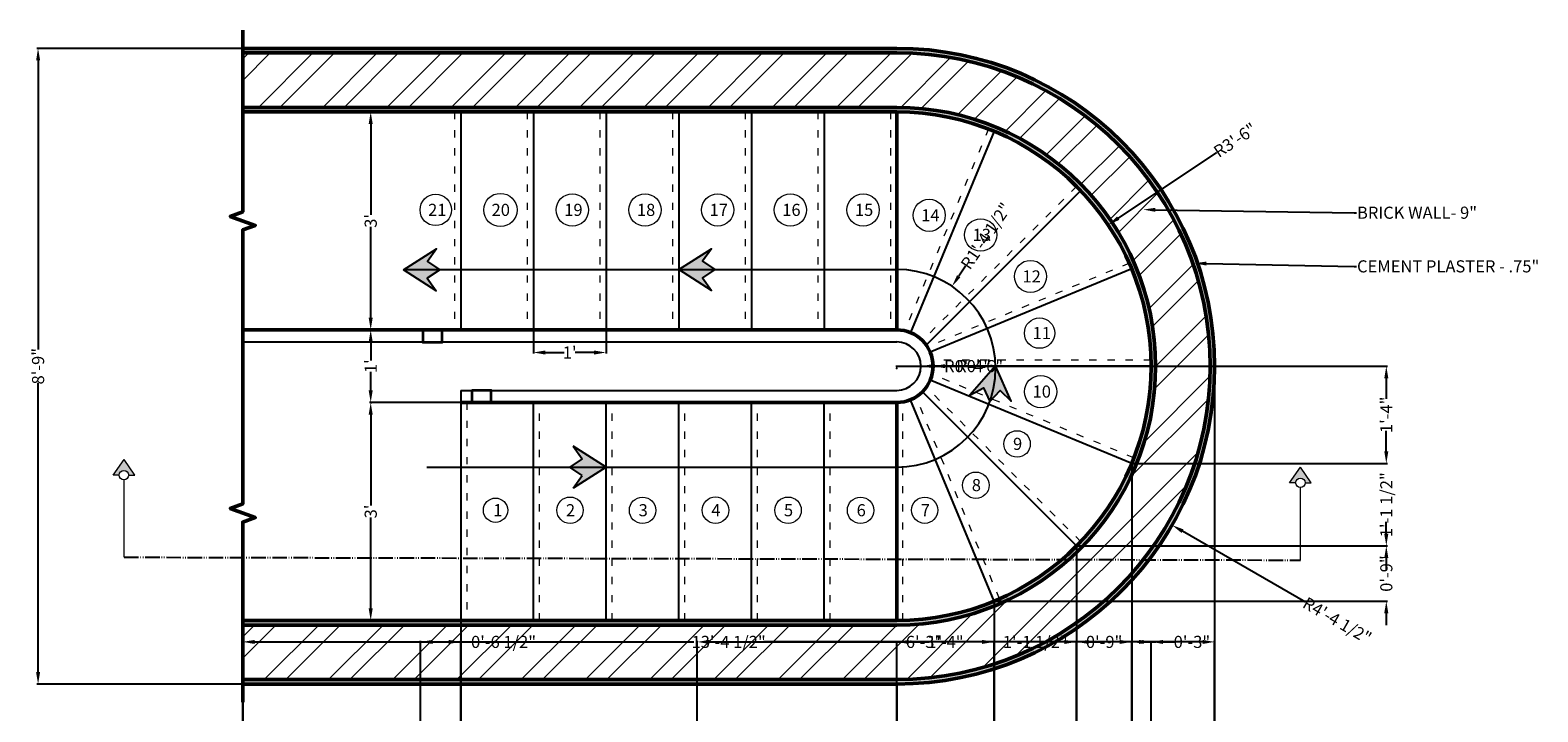
# Model space of a CAD drawing. Units: inches. Extents: x 865 to 1137, y 672 to 989.
# Tile 3 of 3: x 885 to 1134, y 876 to 989. Entities that reach past the tile are written whole.
import ezdxf
from ezdxf import colors
from ezdxf.entities.mleader import LeaderData, LeaderLine
from ezdxf.math import Vec2, Vec3

# ---------------------------------------------------------------- set-up
doc = ezdxf.new("R2010")
doc.units = ezdxf.units.IN
doc.header["$LTSCALE"] = 0.1
doc.header["$MEASUREMENT"] = 0
doc.linetypes.add('ACAD_ISO03W100', pattern=[30, 12, -18])
doc.linetypes.add('ACAD_ISO05W100', pattern=[33, 24, -3, 0, -3, 0, -3])
for name, color, linetype, lineweight in [('A-ANNO-DIMS', 2, 'Continuous', 18), ('A-ANNO-SECT', 1, 'ACAD_ISO05W100', 25), ('A-ANNO-SYMB', 3, 'Continuous', 18), ('A-ANNO-TEXT', 3, 'Continuous', 18), ('A-FLOR-STRS', 4, 'Continuous', 25), ('A-FLOR-STRS-NOSG', 4, 'ACAD_ISO03W100', 18), ('A-WALL', 7, 'Continuous', 50), ('A-WALL-PATT', 8, 'Continuous', 18)]:
    doc.layers.add(name, color=color, linetype=linetype, lineweight=lineweight)
doc.styles.get("Standard").update_dxf_attribs({"font": 'arial.ttf', "height": 2})
doc.dimstyles.get("Standard").update_dxf_attribs({"dimtxt": 2, "dimasz": 2, "dimexe": 0.18, "dimexo": 0.0625, "dimgap": 0.09, "dimtad": 0, "dimdec": 0, "dimzin": 0, "dimdsep": 46, "dimlunit": 3, "dimtxsty": 'Standard', "dimcen": 0.09, "dimadec": 0, "dimazin": 0, "dimtfac": 1, "dimtdec": 0, "dimtofl": 0, "dimtmove": 0, "dimatfit": 3, "dimfxl": 1, "dimtolj": 1, "dimtzin": 0, "dimarcsym": 0})

# ---------------------------------------------------------------- blocks, each defined once
blk = doc.blocks.new('*D1')
at = {"layer": 'A-ANNO-DIMS', "color": 0, "lineweight": -2, "transparency": 16777216}
for p, q in [((956.3, 927.25), (941.32, 927.25)), ((941.5, 925.25), (941.5, 910.26)), ((941.5, 893.25), (941.5, 908.25)), ((956.3, 891.25), (941.32, 891.25))]:
    blk.add_line(p, q, dxfattribs=at)
at = {"layer": 'A-ANNO-DIMS', "color": 0, "transparency": 16777216}
for points in [[(941.16, 925.25), (941.83, 925.25), (941.5, 927.25)], [(941.16, 893.25), (941.83, 893.25), (941.5, 891.25)]]:
    blk.add_solid(points, dxfattribs=at)
at = {"layer": 'Defpoints', "color": 0, "transparency": 16777216}
for p in [(941.5, 927.25), (956.36, 927.25), (956.36, 891.25)]:
    blk.add_point(p, dxfattribs=at)
at = {"layer": 'A-ANNO-DIMS', "color": 0, "transparency": 16777216, "insert": (941.5, 909.25), "char_height": 2, "attachment_point": 5, "rotation": 90}
blk.add_mtext("\\A1;3'", dxfattribs=at)
blk = doc.blocks.new('*D2')
at = {"layer": 'A-ANNO-DIMS', "color": 0, "lineweight": -2, "transparency": 16777216}
for p, q in [((941.56, 939.25), (941.68, 939.25)), ((941.5, 937.25), (941.5, 934.17)), ((941.5, 929.25), (941.5, 932.34)), ((941.56, 927.25), (941.68, 927.25))]:
    blk.add_line(p, q, dxfattribs=at)
at = {"layer": 'A-ANNO-DIMS', "color": 0, "transparency": 16777216}
for points in [[(941.16, 937.25), (941.83, 937.25), (941.5, 939.25)], [(941.16, 929.25), (941.83, 929.25), (941.5, 927.25)]]:
    blk.add_solid(points, dxfattribs=at)
at = {"layer": 'Defpoints', "color": 0, "transparency": 16777216}
for p in [(941.5, 939.25), (941.5, 939.25), (941.5, 927.25)]:
    blk.add_point(p, dxfattribs=at)
at = {"layer": 'A-ANNO-DIMS', "color": 0, "transparency": 16777216, "insert": (941.5, 933.25), "char_height": 2, "attachment_point": 5, "rotation": 90}
blk.add_mtext("\\A1;1'", dxfattribs=at)
blk = doc.blocks.new('*D3')
at = {"layer": 'A-ANNO-DIMS', "color": 0, "lineweight": -2, "transparency": 16777216}
for p, q in [((941.56, 975.25), (941.68, 975.25)), ((941.5, 973.25), (941.5, 958.26)), ((941.5, 941.25), (941.5, 956.25)), ((941.56, 939.25), (941.68, 939.25))]:
    blk.add_line(p, q, dxfattribs=at)
at = {"layer": 'A-ANNO-DIMS', "color": 0, "transparency": 16777216}
for points in [[(941.16, 973.25), (941.83, 973.25), (941.5, 975.25)], [(941.16, 941.25), (941.83, 941.25), (941.5, 939.25)]]:
    blk.add_solid(points, dxfattribs=at)
at = {"layer": 'Defpoints', "color": 0, "transparency": 16777216}
for p in [(941.5, 975.25), (941.5, 975.25), (941.5, 939.25)]:
    blk.add_point(p, dxfattribs=at)
at = {"layer": 'A-ANNO-DIMS', "color": 0, "transparency": 16777216, "insert": (941.5, 957.25), "char_height": 2, "attachment_point": 5, "rotation": 90}
blk.add_mtext("\\A1;3'", dxfattribs=at)
blk = doc.blocks.new('*D4')
at = {"layer": 'A-ANNO-DIMS', "color": 0, "lineweight": -2, "transparency": 16777216}
for p, q in [((968.36, 939.19), (968.36, 935.33)), ((980.36, 939.19), (980.36, 935.33)), ((970.36, 935.51), (973.44, 935.51)), ((978.36, 935.51), (975.27, 935.51))]:
    blk.add_line(p, q, dxfattribs=at)
at = {"layer": 'A-ANNO-DIMS', "color": 0, "transparency": 16777216}
for points in [[(970.36, 935.84), (970.36, 935.17), (968.36, 935.51)], [(978.36, 935.84), (978.36, 935.17), (980.36, 935.51)]]:
    blk.add_solid(points, dxfattribs=at)
at = {"layer": 'Defpoints', "color": 0, "transparency": 16777216}
for p in [(968.36, 939.25), (980.36, 939.25), (980.36, 935.51)]:
    blk.add_point(p, dxfattribs=at)
at = {"layer": 'A-ANNO-DIMS', "color": 0, "transparency": 16777216, "insert": (974.36, 935.51), "char_height": 2, "attachment_point": 5}
blk.add_mtext("\\A1;1'", dxfattribs=at)
blk = doc.blocks.new('SECTION-MARK')
for p, q in [((0, 0.78), (1.79, 3.37)), ((3.56, 0.78), (1.79, 3.37)), ((1, 0.78), (0, 0.78)), ((2.56, 0.78), (3.56, 0.78))]:
    blk.add_line(p, q)
blk.add_circle((1.78, 0.78), 0.781)
blk = doc.blocks.new('*D11')
at = {"layer": 'A-ANNO-DIMS', "color": 0, "lineweight": -2, "transparency": 16777216}
for p, q in [((920.3, 985.75), (886.39, 985.75)), ((886.57, 983.75), (886.57, 936)), ((886.57, 882.75), (886.57, 930.51)), ((920.3, 880.75), (886.39, 880.75))]:
    blk.add_line(p, q, dxfattribs=at)
at = {"layer": 'A-ANNO-DIMS', "color": 0, "transparency": 16777216}
for points in [[(886.24, 983.75), (886.91, 983.75), (886.57, 985.75)], [(886.24, 882.75), (886.91, 882.75), (886.57, 880.75)]]:
    blk.add_solid(points, dxfattribs=at)
at = {"layer": 'Defpoints', "color": 0, "transparency": 16777216}
for p in [(920.36, 985.75), (886.57, 880.75), (920.36, 880.75)]:
    blk.add_point(p, dxfattribs=at)
at = {"layer": 'A-ANNO-DIMS', "color": 0, "transparency": 16777216, "insert": (886.57, 933.25), "char_height": 2, "attachment_point": 5, "rotation": 90}
blk.add_mtext('\\A1;8\'-9"', dxfattribs=at)
blk = doc.blocks.new('*D12')
at = {"layer": 'A-ANNO-DIMS', "color": 0, "lineweight": -2, "transparency": 16777216}
for p, q in [((956.36, 891.19), (956.36, 865.17)), ((920.36, 880.69), (920.36, 865.17)), ((922.36, 865.35), (935.61, 865.35)), ((954.36, 865.35), (941.11, 865.35))]:
    blk.add_line(p, q, dxfattribs=at)
at = {"layer": 'A-ANNO-DIMS', "color": 0, "transparency": 16777216}
for points in [[(922.36, 865.69), (922.36, 865.02), (920.36, 865.35)], [(954.36, 865.69), (954.36, 865.02), (956.36, 865.35)]]:
    blk.add_solid(points, dxfattribs=at)
at = {"layer": 'Defpoints', "color": 0, "transparency": 16777216}
for p in [(956.36, 891.25), (920.36, 880.75), (956.36, 865.35)]:
    blk.add_point(p, dxfattribs=at)
at = {"layer": 'A-ANNO-DIMS', "color": 0, "transparency": 16777216, "insert": (938.36, 865.35), "char_height": 2, "attachment_point": 5}
blk.add_mtext('\\A1;3\'-0"', dxfattribs=at)
blk = doc.blocks.new('*D13')
at = {"layer": 'A-ANNO-DIMS', "color": 0, "lineweight": -2, "transparency": 16777216}
for p, q in [((956.36, 891.19), (956.36, 865.17)), ((1028.36, 880.69), (1028.36, 865.17)), ((958.36, 865.35), (989.6, 865.35)), ((1026.36, 865.35), (995.11, 865.35))]:
    blk.add_line(p, q, dxfattribs=at)
at = {"layer": 'A-ANNO-DIMS', "color": 0, "transparency": 16777216}
for points in [[(958.36, 865.69), (958.36, 865.02), (956.36, 865.35)], [(1026.36, 865.69), (1026.36, 865.02), (1028.36, 865.35)]]:
    blk.add_solid(points, dxfattribs=at)
at = {"layer": 'Defpoints', "color": 0, "transparency": 16777216}
for p in [(956.36, 891.25), (1028.36, 880.75), (1028.36, 865.35)]:
    blk.add_point(p, dxfattribs=at)
at = {"layer": 'A-ANNO-DIMS', "color": 0, "transparency": 16777216, "insert": (992.36, 865.35), "char_height": 2, "attachment_point": 5}
blk.add_mtext('\\A1;6\'-0"', dxfattribs=at)
blk = doc.blocks.new('*D14')
at = {"layer": 'A-ANNO-DIMS', "color": 0, "lineweight": -2, "transparency": 16777216}
for p, q in [((1044.43, 894.39), (1044.43, 865.17)), ((1028.36, 880.69), (1028.36, 865.17)), ((1030.36, 865.35), (1033.74, 865.35)), ((1042.43, 865.35), (1039.05, 865.35))]:
    blk.add_line(p, q, dxfattribs=at)
at = {"layer": 'A-ANNO-DIMS', "color": 0, "transparency": 16777216}
for points in [[(1030.36, 865.69), (1030.36, 865.02), (1028.36, 865.35)], [(1042.43, 865.69), (1042.43, 865.02), (1044.43, 865.35)]]:
    blk.add_solid(points, dxfattribs=at)
at = {"layer": 'Defpoints', "color": 0, "transparency": 16777216}
for p in [(1044.43, 894.45), (1028.36, 880.75), (1044.43, 865.35)]:
    blk.add_point(p, dxfattribs=at)
at = {"layer": 'A-ANNO-DIMS', "color": 0, "transparency": 16777216, "insert": (1036.39, 865.35), "char_height": 2, "attachment_point": 5}
blk.add_mtext('\\A1;1\'-4"', dxfattribs=at)
blk = doc.blocks.new('*D15')
at = {"layer": 'A-ANNO-DIMS', "color": 0, "lineweight": -2, "transparency": 16777216}
for p, q in [((1058.06, 903.49), (1058.06, 865.17)), ((1044.43, 894.39), (1044.43, 865.17)), ((1042.43, 865.35), (1040.43, 865.35)), ((1060.06, 865.35), (1062.06, 865.35))]:
    blk.add_line(p, q, dxfattribs=at)
at = {"layer": 'A-ANNO-DIMS', "color": 0, "transparency": 16777216}
for points in [[(1042.43, 865.69), (1042.43, 865.02), (1044.43, 865.35)], [(1060.06, 865.69), (1060.06, 865.02), (1058.06, 865.35)]]:
    blk.add_solid(points, dxfattribs=at)
at = {"layer": 'Defpoints', "color": 0, "transparency": 16777216}
for p in [(1058.06, 903.56), (1044.43, 894.45), (1058.06, 865.35)]:
    blk.add_point(p, dxfattribs=at)
at = {"layer": 'A-ANNO-DIMS', "color": 0, "transparency": 16777216, "insert": (1051.24, 865.35), "char_height": 2, "attachment_point": 5}
blk.add_mtext('\\A1;1\'-1 1/2"', dxfattribs=at)
blk = doc.blocks.new('*D16')
at = {"layer": 'A-ANNO-DIMS', "color": 0, "lineweight": -2, "transparency": 16777216}
for p, q in [((1067.16, 917.12), (1067.16, 865.17)), ((1058.06, 903.49), (1058.06, 865.17)), ((1056.06, 865.35), (1054.06, 865.35)), ((1069.16, 865.35), (1071.16, 865.35))]:
    blk.add_line(p, q, dxfattribs=at)
at = {"layer": 'A-ANNO-DIMS', "color": 0, "transparency": 16777216}
for points in [[(1056.06, 865.69), (1056.06, 865.02), (1058.06, 865.35)], [(1069.16, 865.69), (1069.16, 865.02), (1067.16, 865.35)]]:
    blk.add_solid(points, dxfattribs=at)
at = {"layer": 'Defpoints', "color": 0, "transparency": 16777216}
for p in [(1067.16, 917.18), (1058.06, 903.56), (1067.16, 865.35)]:
    blk.add_point(p, dxfattribs=at)
at = {"layer": 'A-ANNO-DIMS', "color": 0, "transparency": 16777216, "insert": (1062.61, 865.35), "char_height": 2, "attachment_point": 5}
blk.add_mtext('\\A1;0\'-9"', dxfattribs=at)
blk = doc.blocks.new('*D17')
at = {"layer": 'A-ANNO-DIMS', "color": 0, "lineweight": -2, "transparency": 16777216}
for p, q in [((1080.86, 933.19), (1080.86, 865.17)), ((1067.16, 917.12), (1067.16, 865.17)), ((1065.16, 865.35), (1063.16, 865.35)), ((1082.86, 865.35), (1084.86, 865.35))]:
    blk.add_line(p, q, dxfattribs=at)
at = {"layer": 'A-ANNO-DIMS', "color": 0, "transparency": 16777216}
for points in [[(1065.16, 865.69), (1065.16, 865.02), (1067.16, 865.35)], [(1082.86, 865.69), (1082.86, 865.02), (1080.86, 865.35)]]:
    blk.add_solid(points, dxfattribs=at)
at = {"layer": 'Defpoints', "color": 0, "transparency": 16777216}
for p in [(1080.86, 933.25), (1067.16, 917.18), (1080.86, 865.35)]:
    blk.add_point(p, dxfattribs=at)
at = {"layer": 'A-ANNO-DIMS', "color": 0, "transparency": 16777216, "insert": (1074.01, 865.35), "char_height": 2, "attachment_point": 5}
blk.add_mtext('\\A1;1\'-1 1/2"', dxfattribs=at)
blk = doc.blocks.new('*D18')
at = {"layer": 'A-ANNO-DIMS', "color": 0, "lineweight": -2, "transparency": 16777216}
for p, q in [((1028.42, 933.25), (1109.39, 933.25)), ((1109.21, 931.25), (1109.21, 927.87)), ((1109.21, 919.18), (1109.21, 922.56)), ((1067.22, 917.18), (1109.39, 917.18))]:
    blk.add_line(p, q, dxfattribs=at)
at = {"layer": 'A-ANNO-DIMS', "color": 0, "transparency": 16777216}
for points in [[(1108.87, 931.25), (1109.54, 931.25), (1109.21, 933.25)], [(1108.87, 919.18), (1109.54, 919.18), (1109.21, 917.18)]]:
    blk.add_solid(points, dxfattribs=at)
at = {"layer": 'Defpoints', "color": 0, "transparency": 16777216}
for p in [(1028.36, 933.25), (1067.16, 917.18), (1109.21, 917.18)]:
    blk.add_point(p, dxfattribs=at)
at = {"layer": 'A-ANNO-DIMS', "color": 0, "transparency": 16777216, "insert": (1109.21, 925.22), "char_height": 2, "attachment_point": 5, "rotation": 90}
blk.add_mtext('\\A1;1\'-4"', dxfattribs=at)
blk = doc.blocks.new('*D19')
at = {"layer": 'A-ANNO-DIMS', "color": 0, "lineweight": -2, "transparency": 16777216}
for p, q in [((1109.21, 919.18), (1109.21, 921.18)), ((1067.22, 917.18), (1109.39, 917.18)), ((1058.12, 903.56), (1109.39, 903.56)), ((1109.21, 901.56), (1109.21, 899.56))]:
    blk.add_line(p, q, dxfattribs=at)
at = {"layer": 'A-ANNO-DIMS', "color": 0, "transparency": 16777216}
for points in [[(1108.87, 919.18), (1109.54, 919.18), (1109.21, 917.18)], [(1108.87, 901.56), (1109.54, 901.56), (1109.21, 903.56)]]:
    blk.add_solid(points, dxfattribs=at)
at = {"layer": 'Defpoints', "color": 0, "transparency": 16777216}
for p in [(1067.16, 917.18), (1058.06, 903.56), (1109.21, 903.56)]:
    blk.add_point(p, dxfattribs=at)
at = {"layer": 'A-ANNO-DIMS', "color": 0, "transparency": 16777216, "insert": (1109.21, 910.37), "char_height": 2, "attachment_point": 5, "rotation": 90}
blk.add_mtext('\\A1;1\'-1 1/2"', dxfattribs=at)
blk = doc.blocks.new('*D20')
at = {"layer": 'A-ANNO-DIMS', "color": 0, "lineweight": -2, "transparency": 16777216}
for p, q in [((1109.21, 905.56), (1109.21, 907.56)), ((1058.12, 903.56), (1109.39, 903.56)), ((1044.49, 894.45), (1109.39, 894.45)), ((1109.21, 892.45), (1109.21, 890.45))]:
    blk.add_line(p, q, dxfattribs=at)
at = {"layer": 'A-ANNO-DIMS', "color": 0, "transparency": 16777216}
for points in [[(1108.87, 905.56), (1109.54, 905.56), (1109.21, 903.56)], [(1108.87, 892.45), (1109.54, 892.45), (1109.21, 894.45)]]:
    blk.add_solid(points, dxfattribs=at)
at = {"layer": 'Defpoints', "color": 0, "transparency": 16777216}
for p in [(1058.06, 903.56), (1044.43, 894.45), (1109.21, 894.45)]:
    blk.add_point(p, dxfattribs=at)
at = {"layer": 'A-ANNO-DIMS', "color": 0, "transparency": 16777216, "insert": (1109.21, 899), "char_height": 2, "attachment_point": 5, "rotation": 90}
blk.add_mtext('\\A1;0\'-9"', dxfattribs=at)
blk = doc.blocks.new('*D21')
at = {"layer": 'A-ANNO-DIMS', "color": 0, "lineweight": -2, "transparency": 16777216}
for p, q in [((920.36, 835.61), (920.36, 887.89)), ((922.36, 887.71), (994.85, 887.71)), ((1078.86, 887.71), (1006.37, 887.71)), ((1080.86, 861.4), (1080.86, 887.89))]:
    blk.add_line(p, q, dxfattribs=at)
at = {"layer": 'A-ANNO-DIMS', "color": 0, "transparency": 16777216}
for points in [[(922.36, 888.04), (922.36, 887.37), (920.36, 887.71)], [(1078.86, 888.04), (1078.86, 887.37), (1080.86, 887.71)]]:
    blk.add_solid(points, dxfattribs=at)
at = {"layer": 'Defpoints', "color": 0, "transparency": 16777216}
for p in [(1080.86, 887.71), (1080.86, 861.34), (920.36, 835.55)]:
    blk.add_point(p, dxfattribs=at)
at = {"layer": 'A-ANNO-DIMS', "color": 0, "transparency": 16777216, "insert": (1000.61, 887.71), "char_height": 2, "attachment_point": 5}
blk.add_mtext('\\A1;13\'-4 1/2"', dxfattribs=at)
blk = doc.blocks.new('*D29')
at = {"layer": 'A-ANNO-DIMS', "color": 0, "lineweight": -2, "transparency": 16777216}
for p, q in [((949.74, 835.61), (949.74, 887.89)), ((951.74, 887.71), (954.36, 887.71)), ((956.36, 834.61), (956.36, 887.89)), ((956.36, 887.71), (958.36, 887.71))]:
    blk.add_line(p, q, dxfattribs=at)
at = {"layer": 'A-ANNO-DIMS', "color": 0, "transparency": 16777216}
for points in [[(951.74, 888.04), (951.74, 887.37), (949.74, 887.71)], [(954.36, 888.04), (954.36, 887.37), (956.36, 887.71)]]:
    blk.add_solid(points, dxfattribs=at)
at = {"layer": 'Defpoints', "color": 0, "transparency": 16777216}
for p in [(956.36, 887.71), (949.74, 835.55), (956.36, 834.55)]:
    blk.add_point(p, dxfattribs=at)
at = {"layer": 'A-ANNO-DIMS', "color": 0, "transparency": 16777216, "insert": (963.44, 887.71), "char_height": 2, "attachment_point": 5}
blk.add_mtext('\\A1;0\'-6 1/2"', dxfattribs=at)
blk = doc.blocks.new('*D30')
at = {"layer": 'A-ANNO-DIMS', "color": 0, "lineweight": -2, "transparency": 16777216}
for p, q in [((995.4, 797.55), (995.4, 887.89)), ((997.4, 887.71), (1030.12, 887.71)), ((1068.36, 887.71), (1035.63, 887.71)), ((1070.36, 861.4), (1070.36, 887.89))]:
    blk.add_line(p, q, dxfattribs=at)
at = {"layer": 'A-ANNO-DIMS', "color": 0, "transparency": 16777216}
for points in [[(997.4, 888.04), (997.4, 887.37), (995.4, 887.71)], [(1068.36, 888.04), (1068.36, 887.37), (1070.36, 887.71)]]:
    blk.add_solid(points, dxfattribs=at)
at = {"layer": 'Defpoints', "color": 0, "transparency": 16777216}
for p in [(1070.36, 887.71), (1070.36, 861.34), (995.4, 797.49)]:
    blk.add_point(p, dxfattribs=at)
at = {"layer": 'A-ANNO-DIMS', "color": 0, "transparency": 16777216, "insert": (1032.88, 887.71), "char_height": 2, "attachment_point": 5}
blk.add_mtext('\\A1;6\'-3"', dxfattribs=at)
blk = doc.blocks.new('*D32')
at = {"layer": 'A-ANNO-DIMS', "color": 0, "lineweight": -2, "transparency": 16777216}
for p, q in [((1028.36, 779.61), (1028.36, 887.89)), ((1030.36, 887.71), (1033.74, 887.71)), ((1042.43, 887.71), (1039.05, 887.71)), ((1044.43, 779.61), (1044.43, 887.89))]:
    blk.add_line(p, q, dxfattribs=at)
at = {"layer": 'A-ANNO-DIMS', "color": 0, "transparency": 16777216}
for points in [[(1030.36, 888.04), (1030.36, 887.37), (1028.36, 887.71)], [(1042.43, 888.04), (1042.43, 887.37), (1044.43, 887.71)]]:
    blk.add_solid(points, dxfattribs=at)
at = {"layer": 'Defpoints', "color": 0, "transparency": 16777216}
for p in [(1044.43, 887.71), (1028.36, 779.55), (1044.43, 779.55)]:
    blk.add_point(p, dxfattribs=at)
at = {"layer": 'A-ANNO-DIMS', "color": 0, "transparency": 16777216, "insert": (1036.39, 887.71), "char_height": 2, "attachment_point": 5}
blk.add_mtext('\\A1;1\'-4"', dxfattribs=at)
blk = doc.blocks.new('*D33')
at = {"layer": 'A-ANNO-DIMS', "color": 0, "lineweight": -2, "transparency": 16777216}
for p, q in [((1042.43, 887.71), (1040.43, 887.71)), ((1044.43, 785.61), (1044.43, 887.89)), ((1058.06, 779.61), (1058.06, 887.89)), ((1060.06, 887.71), (1062.06, 887.71))]:
    blk.add_line(p, q, dxfattribs=at)
at = {"layer": 'A-ANNO-DIMS', "color": 0, "transparency": 16777216}
for points in [[(1042.43, 888.04), (1042.43, 887.37), (1044.43, 887.71)], [(1060.06, 888.04), (1060.06, 887.37), (1058.06, 887.71)]]:
    blk.add_solid(points, dxfattribs=at)
at = {"layer": 'Defpoints', "color": 0, "transparency": 16777216}
for p in [(1058.06, 887.71), (1044.43, 785.55), (1058.06, 779.55)]:
    blk.add_point(p, dxfattribs=at)
at = {"layer": 'A-ANNO-DIMS', "color": 0, "transparency": 16777216, "insert": (1051.24, 887.71), "char_height": 2, "attachment_point": 5}
blk.add_mtext('\\A1;1\'-1 1/2"', dxfattribs=at)
blk = doc.blocks.new('*D34')
at = {"layer": 'A-ANNO-DIMS', "color": 0, "lineweight": -2, "transparency": 16777216}
for p, q in [((1056.06, 887.71), (1054.06, 887.71)), ((1058.06, 779.61), (1058.06, 887.89)), ((1067.16, 771.61), (1067.16, 887.89)), ((1069.16, 887.71), (1071.16, 887.71))]:
    blk.add_line(p, q, dxfattribs=at)
at = {"layer": 'A-ANNO-DIMS', "color": 0, "transparency": 16777216}
for points in [[(1056.06, 888.04), (1056.06, 887.37), (1058.06, 887.71)], [(1069.16, 888.04), (1069.16, 887.37), (1067.16, 887.71)]]:
    blk.add_solid(points, dxfattribs=at)
at = {"layer": 'Defpoints', "color": 0, "transparency": 16777216}
for p in [(1067.16, 887.71), (1058.06, 779.55), (1067.16, 771.55)]:
    blk.add_point(p, dxfattribs=at)
at = {"layer": 'A-ANNO-DIMS', "color": 0, "transparency": 16777216, "insert": (1062.61, 887.71), "char_height": 2, "attachment_point": 5}
blk.add_mtext('\\A1;0\'-9"', dxfattribs=at)
blk = doc.blocks.new('*D35')
at = {"layer": 'A-ANNO-DIMS', "color": 0, "lineweight": -2, "transparency": 16777216}
for p, q in [((1065.16, 887.71), (1063.16, 887.71)), ((1067.16, 771.61), (1067.16, 887.89)), ((1070.36, 765.61), (1070.36, 887.89)), ((1072.36, 887.71), (1074.36, 887.71))]:
    blk.add_line(p, q, dxfattribs=at)
at = {"layer": 'A-ANNO-DIMS', "color": 0, "transparency": 16777216}
for points in [[(1065.16, 888.04), (1065.16, 887.37), (1067.16, 887.71)], [(1072.36, 888.04), (1072.36, 887.37), (1070.36, 887.71)]]:
    blk.add_solid(points, dxfattribs=at)
at = {"layer": 'Defpoints', "color": 0, "transparency": 16777216}
for p in [(1070.36, 887.71), (1067.16, 771.55), (1070.36, 765.55)]:
    blk.add_point(p, dxfattribs=at)
at = {"layer": 'A-ANNO-DIMS', "color": 0, "transparency": 16777216, "insert": (1077.11, 887.71), "char_height": 2, "attachment_point": 5}
blk.add_mtext('\\A1;0\'-3"', dxfattribs=at)
blk = doc.blocks.new('*D36')
at = {"layer": 'A-ANNO-DIMS', "color": 0, "lineweight": -2, "transparency": 16777216}
for p, q in [((1028.27, 933.25), (1028.45, 933.25)), ((1028.36, 933.16), (1028.36, 933.34)), ((1095.87, 894.26), (1075.55, 906))]:
    blk.add_line(p, q, dxfattribs=at)
at = {"layer": 'A-ANNO-DIMS', "color": 0, "transparency": 16777216}
blk.add_solid([(1075.72, 906.29), (1075.39, 905.71), (1073.82, 907)], dxfattribs=at)
at = {"layer": 'Defpoints', "color": 0, "transparency": 16777216}
for p in [(1028.36, 933.25), (1073.82, 907)]:
    blk.add_point(p, dxfattribs=at)
at = {"layer": 'A-ANNO-DIMS', "color": 0, "transparency": 16777216, "insert": (1101.1, 891.25), "char_height": 2, "attachment_point": 5, "rotation": 329.993}
blk.add_mtext('\\A1;R4\'-4 1/2"', dxfattribs=at)
blk = doc.blocks.new('*D37')
at = {"layer": 'A-ANNO-DIMS', "color": 0, "lineweight": -2, "transparency": 16777216}
for p, q in [((1081.15, 968.53), (1064.94, 957.7)), ((1028.27, 933.25), (1028.45, 933.25)), ((1028.36, 933.16), (1028.36, 933.34))]:
    blk.add_line(p, q, dxfattribs=at)
at = {"layer": 'A-ANNO-DIMS', "color": 0, "transparency": 16777216}
blk.add_solid([(1064.76, 957.98), (1065.13, 957.42), (1063.28, 956.59)], dxfattribs=at)
at = {"layer": 'Defpoints', "color": 0, "transparency": 16777216}
for p in [(1063.28, 956.59), (1028.36, 933.25)]:
    blk.add_point(p, dxfattribs=at)
at = {"layer": 'A-ANNO-DIMS', "color": 0, "transparency": 16777216, "insert": (1084.23, 970.59), "char_height": 2, "attachment_point": 5, "rotation": 33.7516}
blk.add_mtext('\\A1;R3\'-6"', dxfattribs=at)
blk = doc.blocks.new('*D38')
at = {"layer": 'A-ANNO-DIMS', "color": 0, "lineweight": -2, "transparency": 16777216}
for p, q in [((1039.73, 949.75), (1038.61, 948.1)), ((1028.27, 932.9), (1028.45, 932.9)), ((1028.36, 932.81), (1028.36, 932.99))]:
    blk.add_line(p, q, dxfattribs=at)
at = {"layer": 'A-ANNO-DIMS', "color": 0, "transparency": 16777216}
blk.add_solid([(1038.33, 948.28), (1038.88, 947.91), (1037.49, 946.44)], dxfattribs=at)
at = {"layer": 'Defpoints', "color": 0, "transparency": 16777216}
for p in [(1037.49, 946.44), (1028.36, 932.9)]:
    blk.add_point(p, dxfattribs=at)
at = {"layer": 'A-ANNO-DIMS', "color": 0, "transparency": 16777216, "insert": (1043.1, 954.76), "char_height": 2, "attachment_point": 5, "rotation": 55.9973}
blk.add_mtext('\\A1;R1\'-4 1/2"', dxfattribs=at)
blk = doc.blocks.new('*D39')
at = {"layer": 'A-ANNO-DIMS', "color": 0, "lineweight": -2, "transparency": 16777216}
for p, q in [((1028.27, 933.25), (1028.45, 933.25)), ((1028.36, 933.16), (1028.36, 933.34)), ((1038.36, 933.26), (1036.36, 933.26))]:
    blk.add_line(p, q, dxfattribs=at)
at = {"layer": 'A-ANNO-DIMS', "color": 0, "transparency": 16777216}
blk.add_solid([(1036.36, 933.59), (1036.36, 932.92), (1034.36, 933.25)], dxfattribs=at)
at = {"layer": 'Defpoints', "color": 0, "transparency": 16777216}
for p in [(1028.36, 933.25), (1034.36, 933.25)]:
    blk.add_point(p, dxfattribs=at)
at = {"layer": 'A-ANNO-DIMS', "color": 0, "transparency": 16777216, "insert": (1042.06, 933.26), "char_height": 2, "attachment_point": 5, "rotation": 0.0031}
blk.add_mtext('\\A1;R0\'-6"', dxfattribs=at)
blk = doc.blocks.new('*D40')
at = {"layer": 'A-ANNO-DIMS', "color": 0, "lineweight": -2, "transparency": 16777216}
for p, q in [((1028.27, 933.25), (1028.45, 933.25)), ((1028.36, 933.16), (1028.36, 933.34)), ((1036.36, 933.26), (1034.36, 933.26))]:
    blk.add_line(p, q, dxfattribs=at)
at = {"layer": 'A-ANNO-DIMS', "color": 0, "transparency": 16777216}
blk.add_solid([(1034.36, 933.59), (1034.36, 932.92), (1032.36, 933.25)], dxfattribs=at)
at = {"layer": 'Defpoints', "color": 0, "transparency": 16777216}
for p in [(1028.36, 933.25), (1032.36, 933.25)]:
    blk.add_point(p, dxfattribs=at)
at = {"layer": 'A-ANNO-DIMS', "color": 0, "transparency": 16777216, "insert": (1040.06, 933.26), "char_height": 2, "attachment_point": 5, "rotation": 0.0047}
blk.add_mtext('\\A1;R0\'-4"', dxfattribs=at)

msp = doc.modelspace()

# ---------------------------------------------------------------- hatches: boundary and pattern name
at = {"layer": 'A-ANNO-SYMB'}
h = msp.add_hatch(color=256, dxfattribs=at)
h.dxf.hatch_style = 1
h.paths.add_polyline_path([(952.89, 949.16), (952.79, 949.23), (946.99, 949.23), (946.93, 949.19), (952.32, 945.7), (950.84, 947.79)])
h.paths.add_polyline_path([(950.85, 950.55), (952.35, 952.62), (946.99, 949.23), (952.79, 949.23)])
h.paths.add_polyline_path([(998.32, 949.2), (998.28, 949.23), (992.36, 949.23), (997.75, 945.74), (996.27, 947.83)])
h.paths.add_polyline_path([(996.28, 950.59), (997.78, 952.66), (992.36, 949.23), (998.28, 949.23)])
h.paths.add_polyline_path([(1044.68, 933.25), (1044.59, 933.25), (1040.97, 929.11), (1041.34, 928.96), (1042.71, 929.66), (1043.45, 928.08), (1043.9, 927.9, 0.083443)])
h.paths.add_polyline_path([(1044.68, 933.25, -0.083443), (1043.9, 927.9), (1044.11, 927.81), (1045.43, 929.25), (1047.27, 927.46)])
h.paths.add_polyline_path([(1041.34, 928.96), (1040.97, 929.11), (1040.42, 928.49)])
h.paths.add_polyline_path([(974.95, 920.04), (976.44, 917.95), (974.4, 916.58), (980.36, 916.58)])
h.paths.add_polyline_path([(980.36, 916.58), (974.4, 916.58), (976.44, 915.2), (974.95, 913.12)])
h = msp.add_hatch(color=256, dxfattribs=at)
h.dxf.hatch_style = 1
h.paths.add_polyline_path([(1043.9, 927.9), (1043.45, 928.08), (1043.75, 927.46, 0.007129)])
h.paths.add_polyline_path([(1044.11, 927.81), (1043.9, 927.9, -0.007129), (1043.75, 927.46), (1043.76, 927.43)])
h = msp.add_hatch(color=256, dxfattribs=at)
h.dxf.hatch_style = 1
h.paths.add_polyline_path([(901.54, 915.26), (902.54, 915.26), (900.77, 917.85), (898.97, 915.26), (899.97, 915.26, -1)])
h.paths.add_polyline_path([(1095.04, 916.59), (1093.24, 914), (1094.24, 914, -1), (1095.81, 914), (1096.81, 914)])
at = {"layer": 'A-WALL-PATT'}
h = msp.add_hatch(dxfattribs=at)
h.set_pattern_fill('AR-CONC', color=256, scale=0.3)
h.set_pattern_definition([(50, (0, 0), (2.1517805, -0.1882564), [0.225, -2.475]), (355, (0, 0), (-0.416254, 2.2565764), [0.18, -1.98]), (100.45144, (0.1793, -0.0157), (1.7355265, 2.06832), [0.1912206, -2.1034263]), (46.1842, (0, 0.6), (3.201724, -0.496558), [0.3375, -3.7125]), (96.63564, (0.2668, 0.5586), (2.803986, 2.922356), [0.286831, -3.155141]), (351.18416, (0, 0.6), (2.803986, 2.922356), [0.27, -2.97]), (21, (0.3, 0.45), (1.7907212, -1.2078567), [0.225, -2.475]), (326, (0.3, 0.45), (0.729946, 2.17545), [0.18, -1.98]), (71.45144, (0.4492, 0.3493), (2.520667, 0.9675935), [0.1912206, -2.1034263]), (37.5, (0, 0), (0.03647957, 0.99868156), [0, -1.956, 0, -2.01, 0, -1.9875]), (7.5, (0, 0), (0.7892086, 1.1832351), [0, -1.146, 0, -1.911, 0, -0.7575]), (327.5, (-0.669, 0), (1.6014673, -0.0676646), [0, -0.75, 0, -2.34, 0, -3.105]), (317.5, (-0.969, 0), (1.7495585, 0.300315), [0, -0.975, 0, -1.554, 0, -2.205])])
h.paths.add_polyline_path([(1028.36, 890.5, 1), (1028.36, 976), (920.36, 976), (920.36, 975.25), (1028.36, 975.25, -1), (1028.36, 891.25), (920.36, 891.25), (920.36, 890.5)], flags=17)
h.paths.add_polyline_path([(1028.36, 880.75, 1), (1028.36, 985.75), (920.36, 985.75), (920.36, 985), (1028.36, 985, -1), (1028.36, 881.5), (920.36, 881.5), (920.36, 880.75)])
h = msp.add_hatch(dxfattribs=at)
h.set_pattern_fill('ANSI32', color=256, scale=20)
h.paths.add_polyline_path([(1028.36, 985), (920.36, 985), (920.36, 976), (1028.36, 976, -1), (1028.36, 890.5), (920.36, 890.5), (920.36, 881.5), (1028.36, 881.5, 1)])

# ---------------------------------------------------------------- linework, layer by layer
at = {"layer": 'A-ANNO-SECT'}
msp.add_line((900.76, 901.7), (1095.03, 901.22), dxfattribs=at)
at = {"layer": 'A-ANNO-SYMB'}
for p, q in [((900.76, 901.7), (900.76, 914.48)), ((1095.03, 901.22), (1095.03, 913.22))]:
    msp.add_line(p, q, dxfattribs=at)
for centre, radius in [((952.24, 959.06), 2.59), ((962.91, 959.05), 2.75), ((974.8, 959.05), 2.67), ((986.8, 959.05), 2.67), ((998.8, 959.06), 2.66), ((1010.8, 959.05), 2.67), ((1022.81, 959.05), 2.67), ((1033.73, 958.17), 2.65), ((1042.22, 954.93), 2.67), ((1050.46, 948.08), 2.65), ((1051.95, 938.71), 2.51), ((1052.14, 929.04), 2.67), ((1048.23, 920.4), 2.19), ((1041.42, 913.58), 2.19), ((962.11, 909.46), 2.01), ((974.41, 909.46), 2.18), ((986.4, 909.44), 2.19), ((998.43, 909.46), 2.2), ((1010.41, 909.45), 2.19), ((1022.4, 909.44), 2.19), ((1032.98, 909.46), 2.17)]:
    msp.add_circle(centre, radius, dxfattribs=at)
at = {"layer": 'A-FLOR-STRS'}
for p, q in [((956.36, 975.25), (956.36, 939.25)), ((968.36, 975.25), (968.36, 939.25)), ((980.36, 975.25), (980.36, 939.25)), ((992.36, 975.25), (992.36, 939.25)), ((1004.36, 975.25), (1004.36, 939.25)), ((1016.36, 975.25), (1016.36, 939.25)), ((1044.43, 972.06), (1030.65, 938.8)), ((1058.76, 962.25), (1033.25, 936.73)), ((946.99, 949.23), (1028.36, 949.23)), ((1067.16, 949.33), (1033.9, 935.55)), ((920.36, 937.25), (1028.36, 937.25)), ((1070.36, 933.25), (1034.36, 933.25)), ((956.36, 929.25), (1028.36, 929.25)), ((956.36, 929.25), (956.36, 891.25)), ((1058.06, 903.56), (1032.6, 929.01)), ((1067.16, 917.18), (1033.9, 930.96)), ((968.36, 891.25), (968.36, 927.25)), ((980.36, 891.25), (980.36, 927.25)), ((992.36, 891.25), (992.36, 927.25)), ((1004.36, 891.25), (1004.36, 927.25)), ((1016.36, 891.25), (1016.36, 927.25)), ((1044.43, 894.45), (1030.65, 927.71)), ((980.36, 916.58), (974.95, 920.04)), ((974.95, 920.04), (976.44, 917.95)), ((950.75, 916.58), (1028.36, 916.58)), ((976.44, 917.95), (974.4, 916.58)), ((976.44, 915.2), (974.4, 916.58)), ((980.36, 916.58), (974.95, 913.12)), ((974.95, 913.12), (976.44, 915.2))]:
    msp.add_line(p, q, dxfattribs=at)
for points in [[(946.93, 949.19), (952.35, 952.62), (950.85, 950.55), (952.89, 949.16), (950.84, 947.79), (952.32, 945.7)], [(992.36, 949.23), (997.78, 952.66), (996.28, 950.59), (998.32, 949.2), (996.27, 947.83), (997.75, 945.74)], [(950.1, 939.32), (953.3, 939.32), (953.3, 937.12), (950.1, 937.12)], [(950.2, 939.22), (953.2, 939.22), (953.2, 937.22), (950.2, 937.22)], [(1044.65, 933.33), (1040.42, 928.49), (1042.71, 929.66), (1043.76, 927.43), (1045.43, 929.25), (1047.27, 927.46)], [(958.2, 929.35), (961.4, 929.35), (961.4, 927.15), (958.2, 927.15)], [(958.3, 929.25), (961.3, 929.25), (961.3, 927.25), (958.3, 927.25)]]:
    msp.add_lwpolyline(points, close=True, dxfattribs=at)
for centre, radius in [((1028.36, 932.9), 16.33), ((1028.36, 933.25), 4)]:
    msp.add_arc(centre, radius, 270, 90, dxfattribs=at)
at = {"layer": 'A-FLOR-STRS-NOSG'}
for p, q in [((955.36, 975.25), (955.36, 939.25)), ((967.36, 975.25), (967.36, 939.25)), ((979.36, 975.25), (979.36, 939.25)), ((991.36, 975.25), (991.36, 939.25)), ((1003.36, 975.25), (1003.36, 939.25)), ((1015.36, 975.25), (1015.36, 939.25)), ((1027.36, 975.25), (1027.36, 939.25)), ((1043.51, 972.44), (1029.73, 939.18)), ((1058.06, 962.95), (1032.6, 937.5)), ((1066.78, 950.25), (1033.52, 936.47)), ((1070.36, 934.25), (1034.36, 934.25)), ((1067.54, 918.11), (1034.28, 931.88)), ((1058.76, 904.26), (1033.31, 929.72)), ((957.36, 927.25), (957.36, 891.25)), ((969.36, 891.25), (969.36, 927.25)), ((981.36, 891.25), (981.36, 927.25)), ((993.36, 891.25), (993.36, 927.25)), ((1005.36, 891.25), (1005.36, 927.25)), ((1017.36, 891.25), (1017.36, 927.25)), ((1029.36, 891.25), (1029.36, 927.25)), ((1045.35, 894.83), (1031.58, 928.09))]:
    msp.add_line(p, q, dxfattribs=at)
at = {"layer": 'A-WALL'}
for p, q in [((920.36, 985.75), (1028.36, 985.75)), ((920.36, 985.75), (920.36, 975.25)), ((920.36, 985), (1028.36, 985)), ((920.36, 976), (1028.36, 976)), ((920.36, 975.25), (1028.36, 975.25)), ((1028.36, 975.25), (1028.36, 939.25)), ((1028.36, 975.25), (1028.36, 939.25)), ((920.36, 939.25), (1028.36, 939.25)), ((920.36, 939.25), (920.36, 927.25)), ((956.36, 927.25), (1028.36, 927.25)), ((1028.36, 891.25), (1028.36, 927.25)), ((920.36, 891.25), (1028.36, 891.25)), ((920.36, 891.25), (920.36, 880.75)), ((920.36, 890.5), (1028.36, 890.5)), ((920.36, 881.5), (1028.36, 881.5)), ((920.36, 880.75), (1028.36, 880.75))]:
    msp.add_line(p, q, dxfattribs=at)
for points in [[(920.36, 936.25), (920.36, 955.75), (922.42, 956.5), (918.3, 958), (920.36, 958.75), (920.36, 988.75)], [(920.36, 877.75), (920.36, 907.5), (922.42, 908.25), (918.3, 909.75), (920.36, 910.5), (920.36, 940.25)]]:
    msp.add_lwpolyline(points, dxfattribs=at)
for radius in [52.5, 51.75, 42.75, 42, 6]:
    msp.add_arc((1028.36, 933.25), radius, 270, 90, dxfattribs=at)

# ---------------------------------------------------------------- block references
at = {"layer": 'A-ANNO-SYMB'}
for p in [(898.97, 914.48), (1093.24, 913.22)]:
    msp.add_blockref('SECTION-MARK', p, dxfattribs=at)

# ---------------------------------------------------------------- texts
at = {"layer": 'A-ANNO-TEXT', "char_height": 2, "attachment_point": 1}
for s, width, insert in [('21', 2, (950.98, 960.07)), ('20', 1.0762, (961.46, 960.07)), ('19', 1.0762, (973.46, 960.07)), ('18', 1.0762, (985.46, 960.07)), ('17', 1.0762, (997.46, 960.07)), ('16', 1.0762, (1009.46, 960.07)), ('15', 1.0762, (1021.46, 960.07)), ('14', 1.0762, (1032.4, 959.17)), ('13', 1.0762, (1040.89, 955.95)), ('12', 1.0762, (1049.13, 949.08)), ('11', 1.0762, (1050.8, 939.72)), ('10', 1.0762, (1050.8, 930.06)), ('9', 1.0762, (1047.57, 921.42)), ('8', 1.0762, (1040.76, 914.61)), ('1', 1.0762, (961.74, 910.46)), ('2', 1.0762, (973.74, 910.46)), ('3', 1.0762, (985.74, 910.46)), ('4', 1.0762, (997.74, 910.46)), ('5', 1.0762, (1009.74, 910.46)), ('6', 1.0762, (1021.74, 910.46)), ('7', 1.0762, (1032.33, 910.46))]:
    msp.add_mtext_dynamic_manual_height_columns(s, width=width, gutter_width=10, heights=[0], dxfattribs=dict(at, insert=insert))

# ---------------------------------------------------------------- dimensions: what is measured, and where the dimension line sits
at = {"layer": 'A-ANNO-DIMS'}
for base, p1, p2, override, picture, middle in [((886.57, 880.75), (920.36, 985.75), (920.36, 880.75), {"dimdec": 1, "dimlfac": 1, "dimrnd": 0, "dimzin": 1, "dimdsep": 46, "dimlunit": 4, "dimfrac": 2}, '*D11', (886.57, 933.25)), ((941.5, 975.25), (941.5, 939.25), (941.5, 975.25), {"dimclrd": 0, "dimclre": 0, "dimclrt": 0}, '*D3', (941.5, 957.25)), ((941.5, 939.25), (941.5, 927.25), (941.5, 939.25), {"dimclrd": 0, "dimclre": 0, "dimclrt": 0}, '*D2', (941.5, 933.25)), ((1109.21, 917.18), (1028.36, 933.25), (1067.16, 917.18), {"dimdec": 1, "dimlfac": 1, "dimrnd": 0, "dimzin": 1, "dimdsep": 46, "dimlunit": 4, "dimfrac": 2}, '*D18', (1109.21, 925.22)), ((941.5, 927.25), (956.36, 891.25), (956.36, 927.25), {"dimclrd": 0, "dimclre": 0, "dimclrt": 0}, '*D1', (941.5, 909.25)), ((1109.21, 903.56), (1067.16, 917.18), (1058.06, 903.56), {"dimdec": 1, "dimlfac": 1, "dimrnd": 0, "dimzin": 1, "dimdsep": 46, "dimlunit": 4, "dimfrac": 2}, '*D19', (1109.21, 910.37)), ((1109.21, 894.45), (1058.06, 903.56), (1044.43, 894.45), {"dimdec": 1, "dimlfac": 1, "dimrnd": 0, "dimzin": 1, "dimdsep": 46, "dimlunit": 4, "dimfrac": 2}, '*D20', (1109.21, 899))]:
    dim = msp.add_linear_dim(base=base, p1=p1, p2=p2, angle=90, dimstyle='Standard', override=override, dxfattribs=at)
    dim.commit()
    dim.dimension.update_dxf_attribs({"geometry": picture, "text_midpoint": middle})
for mpoint, picture, middle in [((1063.28, 956.59), '*D37', (1084.23, 970.59)), ((1073.82, 907), '*D36', (1101.1, 891.25))]:
    dim = msp.add_radius_dim(center=(1028.36, 933.25), mpoint=mpoint, dimstyle='Standard', override={"dimdec": 1, "dimlfac": 1, "dimrnd": 0, "dimzin": 1, "dimdsep": 46, "dimlunit": 4, "dimfrac": 2}, dxfattribs=at)
    dim.commit()
    dim.dimension.update_dxf_attribs({"geometry": picture, "text_midpoint": middle, "dimtype": 164})
for center, mpoint, picture, middle in [((1028.36, 932.9), (1037.49, 946.44), '*D38', (1043.1, 954.76)), ((1028.36, 933.25), (1034.36, 933.25), '*D39', (1042.06, 933.26)), ((1028.36, 933.25), (1032.36, 933.25), '*D40', (1040.06, 933.26))]:
    dim = msp.add_radius_dim(center=center, mpoint=mpoint, dimstyle='Standard', override={"dimdec": 1, "dimlfac": 1, "dimrnd": 0, "dimzin": 1, "dimdsep": 46, "dimlunit": 4, "dimfrac": 2}, dxfattribs=at)
    dim.commit()
    dim.dimension.update_dxf_attribs({"geometry": picture, "text_midpoint": middle})
for base, p1, p2, override, picture, middle in [((980.36, 935.51), (968.36, 939.25), (980.36, 939.25), {"dimclrd": 0, "dimclre": 0, "dimclrt": 0}, '*D4', (974.36, 935.51)), ((1080.86, 865.35), (1067.16, 917.18), (1080.86, 933.25), {"dimdec": 1, "dimlfac": 1, "dimrnd": 0, "dimzin": 1, "dimdsep": 46, "dimlunit": 4, "dimfrac": 2}, '*D17', (1074.01, 865.35)), ((1067.16, 865.35), (1058.06, 903.56), (1067.16, 917.18), {"dimdec": 1, "dimlfac": 1, "dimrnd": 0, "dimzin": 1, "dimdsep": 46, "dimlunit": 4, "dimfrac": 2}, '*D16', (1062.61, 865.35)), ((1058.06, 865.35), (1044.43, 894.45), (1058.06, 903.56), {"dimdec": 1, "dimlfac": 1, "dimrnd": 0, "dimzin": 1, "dimdsep": 46, "dimlunit": 4, "dimfrac": 2}, '*D15', (1051.24, 865.35)), ((1044.43, 865.35), (1028.36, 880.75), (1044.43, 894.45), {"dimdec": 1, "dimlfac": 1, "dimrnd": 0, "dimzin": 1, "dimdsep": 46, "dimlunit": 4, "dimfrac": 2}, '*D14', (1036.39, 865.35)), ((956.36, 865.35), (920.36, 880.75), (956.36, 891.25), {"dimdec": 1, "dimlfac": 1, "dimrnd": 0, "dimzin": 1, "dimdsep": 46, "dimlunit": 4, "dimfrac": 2}, '*D12', (938.36, 865.35)), ((1080.86, 887.71), (920.36, 835.55), (1080.86, 861.34), {"dimdec": 1, "dimlfac": 1, "dimrnd": 0, "dimzin": 1, "dimdsep": 46, "dimlunit": 4, "dimfrac": 2}, '*D21', (1000.61, 887.71)), ((956.36, 887.71), (949.74, 835.55), (956.36, 834.55), {"dimdec": 1, "dimlfac": 1, "dimrnd": 0, "dimzin": 1, "dimdsep": 46, "dimlunit": 4, "dimfrac": 2}, '*D29', (963.44, 887.71)), ((1028.36, 865.35), (956.36, 891.25), (1028.36, 880.75), {"dimdec": 1, "dimlfac": 1, "dimrnd": 0, "dimzin": 1, "dimdsep": 46, "dimlunit": 4, "dimfrac": 2}, '*D13', (992.36, 865.35)), ((1070.36, 887.71), (995.4, 797.49), (1070.36, 861.34), {"dimdec": 1, "dimlfac": 1, "dimrnd": 0, "dimzin": 1, "dimdsep": 46, "dimlunit": 4, "dimfrac": 2}, '*D30', (1032.88, 887.71)), ((1044.43, 887.71), (1028.36, 779.55), (1044.43, 779.55), {"dimdec": 1, "dimlfac": 1, "dimrnd": 0, "dimzin": 1, "dimdsep": 46, "dimlunit": 4, "dimfrac": 2}, '*D32', (1036.39, 887.71)), ((1058.06, 887.71), (1044.43, 785.55), (1058.06, 779.55), {"dimdec": 1, "dimlfac": 1, "dimrnd": 0, "dimzin": 1, "dimdsep": 46, "dimlunit": 4, "dimfrac": 2}, '*D33', (1051.24, 887.71)), ((1067.16, 887.71), (1058.06, 779.55), (1067.16, 771.55), {"dimdec": 1, "dimlfac": 1, "dimrnd": 0, "dimzin": 1, "dimdsep": 46, "dimlunit": 4, "dimfrac": 2}, '*D34', (1062.61, 887.71)), ((1070.36, 887.71), (1067.16, 771.55), (1070.36, 765.55), {"dimdec": 1, "dimlfac": 1, "dimrnd": 0, "dimzin": 1, "dimdsep": 46, "dimlunit": 4, "dimfrac": 2}, '*D35', (1077.11, 887.71))]:
    dim = msp.add_linear_dim(base=base, p1=p1, p2=p2, dimstyle='Standard', override=override, dxfattribs=at)
    dim.commit()
    dim.dimension.update_dxf_attribs({"geometry": picture, "text_midpoint": middle})

# ---------------------------------------------------------------- leaders
at = {"layer": 'A-ANNO-TEXT'}
ml = msp.add_multileader_mtext('Standard', dxfattribs=at)
ml.set_content('BRICK WALL- 9"', color=256)
ml.set_leader_properties()
ml.build(insert=Vec2(0, 0))
ml.multileader.update_dxf_attribs({"dogleg_length": 0.36, "arrow_head_size": 2})
ctx = ml.context
ctx.base_point, ctx.char_height, ctx.arrow_head_size, ctx.landing_gap_size, ctx.plane_origin = Vec3(1104.28, 958.58), 2, 2, 0.09, Vec3(1069.06, 959.11)
notes = []
notes.append((ctx, [(0, (1, 1, 0), (1103.92, 958.58), (1, 0), 0.36, [(0, [(1069.06, 959.11)], 0, [])])]))
ctx.mtext.insert, ctx.mtext.flow_direction = Vec3(1104.37, 959.6), 5
ml = msp.add_multileader_mtext('Standard', dxfattribs=at)
ml.set_content('CEMENT PLASTER - .75"', color=256)
ml.set_leader_properties()
ml.build(insert=Vec2(0, 0))
ml.multileader.update_dxf_attribs({"dogleg_length": 0.36, "arrow_head_size": 2})
ctx = ml.context
ctx.base_point, ctx.char_height, ctx.arrow_head_size, ctx.landing_gap_size, ctx.plane_origin = Vec3(1104.28, 949.72), 2, 2, 0.09, Vec3(1077.51, 950.24)
notes.append((ctx, [(0, (1, 1, 0), (1103.92, 949.72), (1, 0), 0.36, [(0, [(1077.51, 950.24)], 0, [])])]))
ctx.mtext.insert, ctx.mtext.flow_direction = Vec3(1104.37, 950.74), 5
for ctx, leaders in notes:
    for number, flags, end, landing, length, lines in leaders:
        leader = LeaderData()
        leader.index, (leader.has_last_leader_line, leader.has_dogleg_vector, leader.attachment_direction) = number, flags
        leader.last_leader_point, leader.dogleg_vector, leader.dogleg_length = Vec3(end), Vec3(landing), length
        for number, points, colour, breaks in lines:
            line = LeaderLine()
            line.index, line.vertices, line.color, line.breaks = number, Vec3.list(points), colors.encode_raw_color(colour), breaks
            leader.lines.append(line)
        ctx.leaders.append(leader)

doc.saveas('drawing.dxf')
